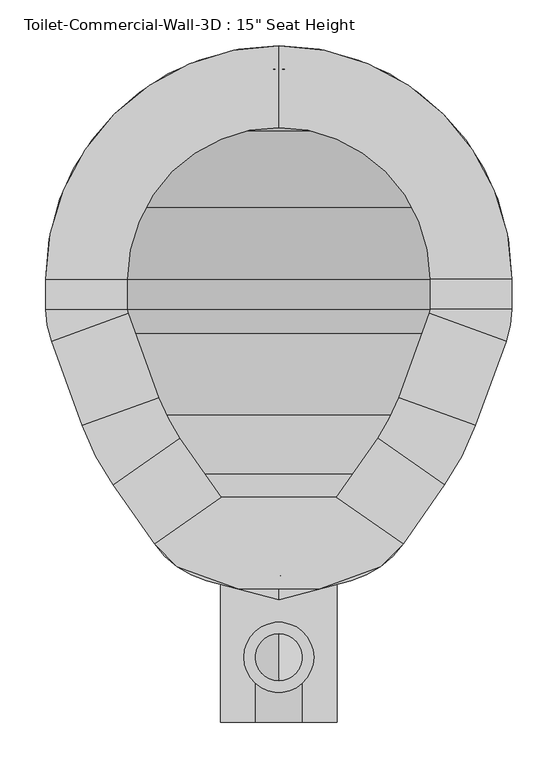
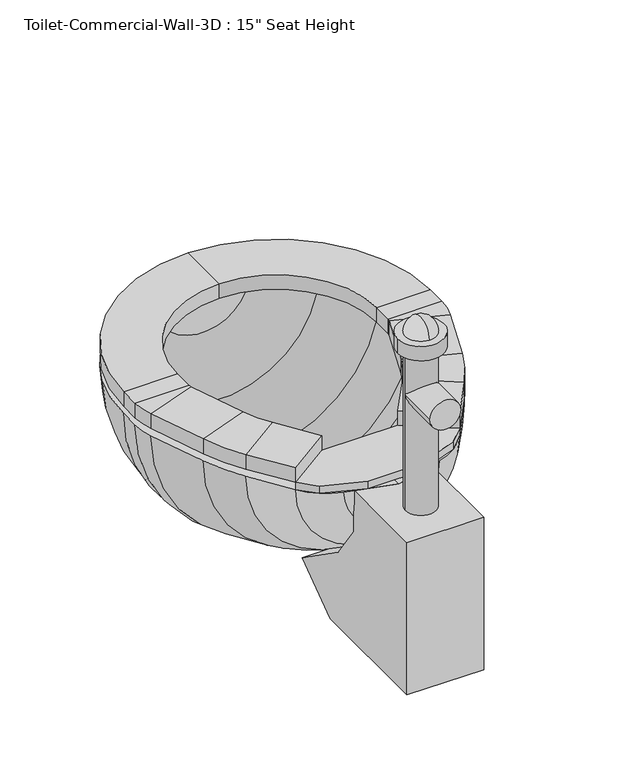
"""IFC4 building model written with IfcOpenShell, lengths in millimetres: flow terminal geometry."""

from ifc_helpers import new_model, si_unit, point, frame, frame_2d, origin, place, context, project, spatial, polyline, circle_curve, ellipse_curve, trimmed, segment, composite_curve, outline, extrude, source, transform, mapped, element, save
from ifc_brep_helpers import plane_surface, cylinder_surface, revolved_surface, advanced_brep


def flow_terminal_bd37145e(model_context):
    return source(origin(), model_context, "Body", "SolidModel", [
        extrude(outline(polyline([(467.7541169, 346.6347495), (540.5767337, 295.6438043), (515.6262519, 270.6933226), (449.563909, 246.6485961), (360.2423986, 246.6485961), (294.1800557, 270.6933226), (269.229574, 295.6438043), (342.0521907, 346.6347495), (467.7541169, 346.6347495)])), frame((0.0, 0.0, 342.9), z_axis=(0.0, 0.0, 1.0), x_axis=(1.0, 0.0, 0.0)), (0.0, 0.0, 1.0), 12.7),
        advanced_brep(
        [(467.7541169, 346.6347495, 355.6), (540.5767337, 295.6438043, 355.6), (540.5767337, 295.6438043, 381.0), (467.7541169, 346.6347495, 381.0), (512.8583992, 411.0503403, 355.6), (585.6810159, 360.0593951, 355.6), (585.6810159, 360.0593951, 381.0), (512.8583992, 411.0503403, 381.0), (619.360053, 424.7562234, 355.6), (535.821379, 455.1618141, 355.6), (619.360053, 424.7562234, 381.0), (535.821379, 455.1618141, 381.0), (569.2372501, 546.9711654, 355.6), (652.7759241, 516.5655747, 355.6), (652.7759241, 516.5655747, 381.0), (569.2372501, 546.9711654, 381.0), (658.9031538, 551.3148212, 355.6), (570.0031538, 551.3148212, 355.6), (658.9031538, 551.3148212, 381.0), (570.0031538, 551.3148212, 381.0), (570.0031538, 584.2, 355.6), (658.9031538, 584.2, 355.6), (658.9031538, 584.2, 381.0), (570.0031538, 584.2, 381.0), (404.9031538, 838.2, 355.6), (404.9031538, 749.3, 355.6), (404.9031538, 838.2, 381.0), (404.9031538, 749.3, 381.0), (150.9031538, 584.2, 355.6), (239.8031538, 584.2, 355.6), (150.9031538, 584.2, 381.0), (239.8031538, 584.2, 381.0), (239.8031538, 551.3148212, 355.6), (150.9031538, 551.3148212, 355.6), (150.9031538, 551.3148212, 381.0), (239.8031538, 551.3148212, 381.0), (157.0303835, 516.5655747, 355.6), (240.5690575, 546.9711654, 355.6), (157.0303835, 516.5655747, 381.0), (240.5690575, 546.9711654, 381.0), (273.9849286, 455.1618141, 355.6), (190.4462546, 424.7562234, 355.6), (190.4462546, 424.7562234, 381.0), (273.9849286, 455.1618141, 381.0), (224.1252917, 360.0593951, 355.6), (296.9479084, 411.0503403, 355.6), (224.1252917, 360.0593951, 381.0), (296.9479084, 411.0503403, 381.0), (342.0521907, 346.6347495, 355.6), (342.0521907, 346.6347495, 381.0), (269.229574, 295.6438043, 381.0), (269.229574, 295.6438043, 355.6)],
        [
            (0, 1),
            (1, 2),
            (2, 3),
            (3, 0),
            (0, 4),
            (4, 5),
            (5, 1),
            (5, 6),
            (6, 2),
            (6, 7),
            (7, 3),
            (7, 4),
            (8, 5, circle_curve(frame((356.8099347, 520.3166514, 355.6), z_axis=(0.0, 0.0, -1.0), x_axis=(0.81915204428899, -0.5735764363510486, 0.0)), 279.4)),
            (4, 9, circle_curve(frame((356.8099347, 520.3166514, 355.6), z_axis=(0.0, 0.0, 1.0), x_axis=(0.81915204428899, -0.5735764363510486, 0.0)), 190.5)),
            (9, 8),
            (10, 6, circle_curve(frame((356.8099347, 520.3166514, 381.0), z_axis=(0.0, 0.0, -1.0), x_axis=(0.81915204428899, -0.5735764363510486, 0.0)), 279.4)),
            (8, 10),
            (11, 7, circle_curve(frame((356.8099347, 520.3166514, 381.0), z_axis=(0.0, 0.0, -1.0), x_axis=(0.81915204428899, -0.5735764363510486, 0.0)), 190.5)),
            (10, 11),
            (11, 9),
            (9, 12),
            (12, 13),
            (13, 8),
            (13, 14),
            (14, 10),
            (14, 15),
            (15, 11),
            (15, 12),
            (16, 13, circle_curve(frame((557.3031538, 551.3148212, 355.6), z_axis=(0.0, 0.0, -1.0), x_axis=(0.939692620785906, -0.34202014332567526, 0.0)), 101.6)),
            (12, 17, circle_curve(frame((557.3031538, 551.3148212, 355.6), z_axis=(0.0, 0.0, 1.0), x_axis=(0.939692620785906, -0.34202014332567526, 0.0)), 12.7)),
            (17, 16),
            (18, 14, circle_curve(frame((557.3031538, 551.3148212, 381.0), z_axis=(0.0, 0.0, -1.0), x_axis=(0.939692620785906, -0.34202014332567526, 0.0)), 101.6)),
            (16, 18),
            (19, 15, circle_curve(frame((557.3031538, 551.3148212, 381.0), z_axis=(0.0, 0.0, -1.0), x_axis=(0.939692620785906, -0.34202014332567526, 0.0)), 12.7)),
            (18, 19),
            (19, 17),
            (17, 20),
            (20, 21),
            (21, 16),
            (21, 22),
            (22, 18),
            (22, 23),
            (23, 19),
            (23, 20),
            (24, 21, circle_curve(frame((404.9031538, 584.2, 355.6), z_axis=(0.0, 0.0, -1.0), x_axis=(1.0, 0.0, 0.0)), 254.0)),
            (20, 25, circle_curve(frame((404.9031538, 584.2, 355.6), z_axis=(0.0, 0.0, 1.0), x_axis=(1.0, 0.0, 0.0)), 165.1)),
            (25, 24),
            (26, 22, circle_curve(frame((404.9031538, 584.2, 381.0), z_axis=(0.0, 0.0, -1.0), x_axis=(1.0, 0.0, 0.0)), 254.0)),
            (24, 26),
            (27, 23, circle_curve(frame((404.9031538, 584.2, 381.0), z_axis=(0.0, 0.0, -1.0), x_axis=(1.0, 0.0, 0.0)), 165.1)),
            (26, 27),
            (27, 25),
            (28, 24, circle_curve(frame((404.9031538, 584.2, 355.6), z_axis=(0.0, 0.0, -1.0), x_axis=(0.0, 1.0, 0.0)), 254.0)),
            (25, 29, circle_curve(frame((404.9031538, 584.2, 355.6), z_axis=(0.0, 0.0, 1.0), x_axis=(0.0, 1.0, 0.0)), 165.1)),
            (29, 28),
            (30, 26, circle_curve(frame((404.9031538, 584.2, 381.0), z_axis=(0.0, 0.0, -1.0), x_axis=(0.0, 1.0, 0.0)), 254.0)),
            (28, 30),
            (31, 27, circle_curve(frame((404.9031538, 584.2, 381.0), z_axis=(0.0, 0.0, -1.0), x_axis=(0.0, 1.0, 0.0)), 165.1)),
            (30, 31),
            (31, 29),
            (29, 32),
            (32, 33),
            (33, 28),
            (33, 34),
            (34, 30),
            (34, 35),
            (35, 31),
            (35, 32),
            (36, 33, circle_curve(frame((252.5031538, 551.3148212, 355.6), z_axis=(0.0, 0.0, -1.0), x_axis=(-1.0, 0.0, 0.0)), 101.6)),
            (32, 37, circle_curve(frame((252.5031538, 551.3148212, 355.6), z_axis=(0.0, 0.0, 1.0), x_axis=(-1.0, 0.0, 0.0)), 12.7)),
            (37, 36),
            (38, 34, circle_curve(frame((252.5031538, 551.3148212, 381.0), z_axis=(0.0, 0.0, -1.0), x_axis=(-1.0, 0.0, 0.0)), 101.6)),
            (36, 38),
            (39, 35, circle_curve(frame((252.5031538, 551.3148212, 381.0), z_axis=(0.0, 0.0, -1.0), x_axis=(-1.0, 0.0, 0.0)), 12.7)),
            (38, 39),
            (39, 37),
            (37, 40),
            (40, 41),
            (41, 36),
            (41, 42),
            (42, 38),
            (42, 43),
            (43, 39),
            (43, 40),
            (44, 41, circle_curve(frame((452.9963729, 520.3166514, 355.6), z_axis=(0.0, 0.0, -1.0), x_axis=(-0.9396926207859088, -0.34202014332566766, 0.0)), 279.4)),
            (40, 45, circle_curve(frame((452.9963729, 520.3166514, 355.6), z_axis=(0.0, 0.0, 1.0), x_axis=(-0.9396926207859088, -0.34202014332566766, 0.0)), 190.5)),
            (45, 44),
            (46, 42, circle_curve(frame((452.9963729, 520.3166514, 381.0), z_axis=(0.0, 0.0, -1.0), x_axis=(-0.9396926207859088, -0.34202014332566766, 0.0)), 279.4)),
            (44, 46),
            (47, 43, circle_curve(frame((452.9963729, 520.3166514, 381.0), z_axis=(0.0, 0.0, -1.0), x_axis=(-0.9396926207859088, -0.34202014332566766, 0.0)), 190.5)),
            (46, 47),
            (47, 45),
            (48, 49),
            (49, 50),
            (50, 51),
            (51, 48),
            (45, 48),
            (51, 44),
            (50, 46),
            (49, 47),
        ],
        [
            plane_surface(frame((540.5767337, 295.6438043, 439.6203184), z_axis=(-0.5735764363510379, -0.8191520442889975, 0.0), x_axis=(0.8191520442889975, -0.5735764363510379, 0.0))),
            plane_surface(frame((467.7541169, 346.6347495, 355.6), z_axis=(0.0, 0.0, -1.0), x_axis=(0.5735764363510375, 0.8191520442889978, 0.0))),
            plane_surface(frame((540.5767337, 295.6438043, 355.6), z_axis=(0.8191520442889973, -0.5735764363510383, 0.0), x_axis=(0.5735764363510383, 0.8191520442889973, 0.0))),
            plane_surface(frame((540.5767337, 295.6438043, 381.0), z_axis=(0.0, 0.0, 1.0), x_axis=(0.573576436351038, 0.8191520442889975, 0.0))),
            plane_surface(frame((467.7541169, 346.6347495, 381.0), z_axis=(-0.8191520442889981, 0.5735764363510371, 0.0), x_axis=(0.5735764363510371, 0.8191520442889981, 0.0))),
            plane_surface(frame((356.8099347, 520.3166514, 355.6), z_axis=(0.0, 0.0, -1.0), x_axis=(0.81915204428899, -0.5735764363510486, 0.0))),
            cylinder_surface(frame((356.8099347, 520.3166514, 342.9), z_axis=(0.0, 0.0, 1.0), x_axis=(0.81915204428899, -0.5735764363510486, 0.0)), 279.4),
            plane_surface(frame((356.8099347, 520.3166514, 381.0), z_axis=(0.0, 0.0, 1.0), x_axis=(0.81915204428899, -0.5735764363510486, 0.0))),
            revolved_surface(polyline([(512.8583991370526, 411.0503402751252, 381.0), (512.8583991370526, 411.0503402751252, 355.6)]), (356.8099347, 520.3166514, 342.9), (0.0, 0.0, 1.0)),
            plane_surface(frame((535.821379, 455.1618141, 355.6), z_axis=(0.0, 0.0, -1.0), x_axis=(0.3420201433256632, 0.9396926207859104, 0.0))),
            plane_surface(frame((619.360053, 424.7562234, 355.6), z_axis=(0.9396926207859108, -0.34202014332566233, 0.0), x_axis=(0.34202014332566233, 0.9396926207859108, 0.0))),
            plane_surface(frame((619.360053, 424.7562234, 381.0), z_axis=(0.0, 0.0, 1.0), x_axis=(0.3420201433256635, 0.9396926207859103, 0.0))),
            plane_surface(frame((535.821379, 455.1618141, 381.0), z_axis=(-0.9396926207859103, 0.3420201433256636, 0.0), x_axis=(0.3420201433256636, 0.9396926207859103, 0.0))),
            plane_surface(frame((557.3031538, 551.3148212, 355.6), z_axis=(0.0, 0.0, -1.0), x_axis=(0.939692620785906, -0.34202014332567526, 0.0))),
            cylinder_surface(frame((557.3031538, 551.3148212, 342.9), z_axis=(0.0, 0.0, 1.0), x_axis=(0.939692620785906, -0.34202014332567526, 0.0)), 101.6),
            plane_surface(frame((557.3031538, 551.3148212, 381.0), z_axis=(0.0, 0.0, 1.0), x_axis=(0.939692620785906, -0.34202014332567526, 0.0))),
            revolved_surface(polyline([(569.237250083981, 546.9711653797639, 381.0), (569.237250083981, 546.9711653797639, 355.6)]), (557.3031538, 551.3148212, 342.9), (0.0, 0.0, 1.0)),
            plane_surface(frame((570.0031538, 551.3148212, 355.6), z_axis=(0.0, 0.0, -1.0), x_axis=(0.0, 1.0, 0.0))),
            plane_surface(frame((658.9031538, 551.3148212, 355.6), z_axis=(1.0, 0.0, 0.0), x_axis=(0.0, 1.0, 0.0))),
            plane_surface(frame((658.9031538, 551.3148212, 381.0), z_axis=(0.0, 0.0, 1.0), x_axis=(0.0, 1.0, 0.0))),
            plane_surface(frame((570.0031538, 551.3148212, 381.0), z_axis=(-1.0, 0.0, 0.0), x_axis=(0.0, 1.0, 0.0))),
            plane_surface(frame((404.9031538, 584.2, 355.6), z_axis=(0.0, 0.0, -1.0), x_axis=(1.0, 0.0, 0.0))),
            cylinder_surface(frame((404.9031538, 584.2, 342.9), z_axis=(0.0, 0.0, 1.0), x_axis=(1.0, 0.0, 0.0)), 254.0),
            plane_surface(frame((404.9031538, 584.2, 381.0), z_axis=(0.0, 0.0, 1.0), x_axis=(1.0, 0.0, 0.0))),
            revolved_surface(polyline([(570.0031538, 584.2, 381.0), (570.0031538, 584.2, 355.6)]), (404.9031538, 584.2, 342.9), (0.0, 0.0, 1.0)),
            plane_surface(frame((404.9031538, 584.2, 355.6), z_axis=(0.0, 0.0, -1.0), x_axis=(0.0, 1.0, 0.0))),
            cylinder_surface(frame((404.9031538, 584.2, 342.9), z_axis=(0.0, 0.0, 1.0), x_axis=(0.0, 1.0, 0.0)), 254.0),
            plane_surface(frame((404.9031538, 584.2, 381.0), z_axis=(0.0, 0.0, 1.0), x_axis=(0.0, 1.0, 0.0))),
            revolved_surface(polyline([(404.9031538, 749.3000000000001, 381.0), (404.9031538, 749.3000000000001, 355.6)]), (404.9031538, 584.2, 342.9), (0.0, 0.0, 1.0)),
            plane_surface(frame((239.8031538, 584.2, 355.6), z_axis=(0.0, 0.0, -1.0), x_axis=(0.0, -1.0, 0.0))),
            plane_surface(frame((150.9031538, 584.2, 355.6), z_axis=(-1.0, 0.0, 0.0), x_axis=(0.0, -1.0, 0.0))),
            plane_surface(frame((150.9031538, 584.2, 381.0), z_axis=(0.0, 0.0, 1.0), x_axis=(0.0, -1.0, 0.0))),
            plane_surface(frame((239.8031538, 584.2, 381.0), z_axis=(1.0, 0.0, 0.0), x_axis=(0.0, -1.0, 0.0))),
            plane_surface(frame((252.5031538, 551.3148212, 355.6), z_axis=(0.0, 0.0, -1.0), x_axis=(-1.0, 0.0, 0.0))),
            cylinder_surface(frame((252.5031538, 551.3148212, 342.9), z_axis=(0.0, 0.0, 1.0), x_axis=(-1.0, 0.0, 0.0)), 101.6),
            plane_surface(frame((252.5031538, 551.3148212, 381.0), z_axis=(0.0, 0.0, 1.0), x_axis=(-1.0, 0.0, 0.0))),
            revolved_surface(polyline([(239.80315380000002, 551.3148212, 381.0), (239.80315380000002, 551.3148212, 355.6)]), (252.5031538, 551.3148212, 342.9), (0.0, 0.0, 1.0)),
            plane_surface(frame((240.5690575, 546.9711654, 355.6), z_axis=(0.0, 0.0, -1.0), x_axis=(0.3420201433256559, -0.9396926207859131, 0.0))),
            plane_surface(frame((157.0303835, 516.5655747, 355.6), z_axis=(-0.9396926207859132, -0.34202014332565567, 0.0), x_axis=(0.34202014332565567, -0.9396926207859132, 0.0))),
            plane_surface(frame((157.0303835, 516.5655747, 381.0), z_axis=(0.0, 0.0, 1.0), x_axis=(0.34202014332565556, -0.9396926207859132, 0.0))),
            plane_surface(frame((240.5690575, 546.9711654, 381.0), z_axis=(0.9396926207859131, 0.34202014332565583, 0.0), x_axis=(0.34202014332565583, -0.9396926207859131, 0.0))),
            plane_surface(frame((452.9963729, 520.3166514, 355.6), z_axis=(0.0, 0.0, -1.0), x_axis=(-0.9396926207859088, -0.34202014332566766, 0.0))),
            cylinder_surface(frame((452.9963729, 520.3166514, 342.9), z_axis=(0.0, 0.0, 1.0), x_axis=(-0.9396926207859088, -0.34202014332566766, 0.0)), 279.4),
            plane_surface(frame((452.9963729, 520.3166514, 381.0), z_axis=(0.0, 0.0, 1.0), x_axis=(-0.9396926207859088, -0.34202014332566766, 0.0))),
            revolved_surface(polyline([(273.98492864028435, 455.16181409646026, 381.0), (273.98492864028435, 455.16181409646026, 355.6)]), (452.9963729, 520.3166514, 342.9), (0.0, 0.0, 1.0)),
            plane_surface(frame((269.229574, 295.6438043, 246.1796816), z_axis=(0.5735764363510504, -0.8191520442889889, 0.0), x_axis=(0.8191520442889889, 0.5735764363510504, 0.0))),
            plane_surface(frame((296.9479084, 411.0503403, 355.6), z_axis=(0.0, 0.0, -1.0000000000000002), x_axis=(0.5735764363510502, -0.819152044288989, 0.0))),
            plane_surface(frame((224.1252917, 360.0593951, 355.6), z_axis=(-0.819152044288989, -0.5735764363510502, 0.0), x_axis=(0.5735764363510502, -0.819152044288989, 0.0))),
            plane_surface(frame((224.1252917, 360.0593951, 381.0), z_axis=(0.0, 0.0, 1.0), x_axis=(0.5735764363510496, -0.8191520442889894, 0.0))),
            plane_surface(frame((296.9479084, 411.0503403, 381.0), z_axis=(0.8191520442889881, 0.5735764363510514, 0.0), x_axis=(0.5735764363510514, -0.8191520442889881, 0.0))),
        ],
        [
            (0, [[1, 2, 3, 4]]),
            (1, [[-1, 5, 6, 7]]),
            (2, [[-2, -7, 8, 9]]),
            (3, [[-3, -9, 10, 11]]),
            (4, [[-4, -11, 12, -5]]),
            (5, [[13, -6, 14, 15]]),
            (6, [[16, -8, -13, 17]]),
            (7, [[18, -10, -16, 19]]),
            (8, [[-14, -12, -18, 20]]),
            (9, [[-15, 21, 22, 23]]),
            (10, [[-17, -23, 24, 25]]),
            (11, [[-19, -25, 26, 27]]),
            (12, [[-20, -27, 28, -21]]),
            (13, [[29, -22, 30, 31]]),
            (14, [[32, -24, -29, 33]]),
            (15, [[34, -26, -32, 35]]),
            (16, [[-30, -28, -34, 36]]),
            (17, [[-31, 37, 38, 39]]),
            (18, [[-33, -39, 40, 41]]),
            (19, [[-35, -41, 42, 43]]),
            (20, [[-36, -43, 44, -37]]),
            (21, [[45, -38, 46, 47]]),
            (22, [[48, -40, -45, 49]]),
            (23, [[50, -42, -48, 51]]),
            (24, [[-46, -44, -50, 52]]),
            (25, [[53, -47, 54, 55]]),
            (26, [[56, -49, -53, 57]]),
            (27, [[58, -51, -56, 59]]),
            (28, [[-54, -52, -58, 60]]),
            (29, [[-55, 61, 62, 63]]),
            (30, [[-57, -63, 64, 65]]),
            (31, [[-59, -65, 66, 67]]),
            (32, [[-60, -67, 68, -61]]),
            (33, [[69, -62, 70, 71]]),
            (34, [[72, -64, -69, 73]]),
            (35, [[74, -66, -72, 75]]),
            (36, [[-70, -68, -74, 76]]),
            (37, [[-71, 77, 78, 79]]),
            (38, [[-73, -79, 80, 81]]),
            (39, [[-75, -81, 82, 83]]),
            (40, [[-76, -83, 84, -77]]),
            (41, [[85, -78, 86, 87]]),
            (42, [[88, -80, -85, 89]]),
            (43, [[90, -82, -88, 91]]),
            (44, [[-86, -84, -90, 92]]),
            (45, [[93, 94, 95, 96]]),
            (46, [[-87, 97, -96, 98]]),
            (47, [[-89, -98, -95, 99]]),
            (48, [[-91, -99, -94, 100]]),
            (49, [[-92, -100, -93, -97]]),
        ],
    ),
        advanced_brep(
        [(491.7762702, 822.8819257, 342.9), (404.9031538, 838.2, 342.9), (404.9031538, 812.8, 342.9), (483.0889586, 799.0137331, 342.9), (566.547764, 745.8446102, 342.9), (619.7168869, 662.3858048, 342.9), (633.5031538, 584.2, 342.9), (633.5031538, 551.3148212, 342.9), (628.9077315, 525.2528863, 342.9), (596.6355667, 436.5858422, 342.9), (562.9565296, 371.8890139, 342.9), (525.0728964, 317.7855786, 342.9), (468.1430637, 277.9228806, 342.9), (404.9031538, 260.9777978, 342.9), (404.9031538, 234.6817829, 342.9), (483.6469009, 255.7811063, 342.9), (540.5767337, 295.6438043, 342.9), (585.6810159, 360.0593951, 342.9), (619.360053, 424.7562234, 342.9), (652.7759241, 516.5655747, 342.9), (658.9031538, 551.3148212, 342.9), (658.9031538, 584.2, 342.9), (643.5850795, 671.0731164, 342.9), (584.5082762, 763.8051224, 342.9), (318.0300374, 822.8819257, 342.9), (225.2980314, 763.8051224, 342.9), (166.2212281, 671.0731164, 342.9), (150.9031538, 584.2, 342.9), (150.9031538, 551.3148212, 342.9), (157.0303835, 516.5655747, 342.9), (190.4462546, 424.7562234, 342.9), (224.1252917, 360.0593951, 342.9), (269.229574, 295.6438043, 342.9), (326.1594067, 255.7811063, 342.9), (341.663244, 277.9228806, 342.9), (284.7334112, 317.7855786, 342.9), (246.849778, 371.8890139, 342.9), (213.1707409, 436.5858422, 342.9), (180.8985761, 525.2528863, 342.9), (176.3031538, 551.3148212, 342.9), (176.3031538, 584.2, 342.9), (190.0894207, 662.3858048, 342.9), (243.2585436, 745.8446102, 342.9), (326.7173491, 799.0137331, 342.9)],
        [
            (0, 1, circle_curve(frame((404.9031538, 584.2, 342.9), z_axis=(0.0, 0.0, 1.0), x_axis=(1.0, 0.0, 0.0)), 254.0)),
            (1, 2),
            (2, 3, circle_curve(frame((404.9031538, 584.2, 342.9), z_axis=(0.0, 0.0, -1.0), x_axis=(1.0, 0.0, 0.0)), 228.6)),
            (3, 4, circle_curve(frame((404.9031538, 584.2, 342.9), z_axis=(0.0, 0.0, -1.0), x_axis=(1.0, 0.0, 0.0)), 228.6)),
            (4, 5, circle_curve(frame((404.9031538, 584.2, 342.9), z_axis=(0.0, 0.0, -1.0), x_axis=(1.0, 0.0, 0.0)), 228.6)),
            (5, 6, circle_curve(frame((404.9031538, 584.2, 342.9), z_axis=(0.0, 0.0, -1.0), x_axis=(1.0, 0.0, 0.0)), 228.6)),
            (6, 7),
            (7, 8, circle_curve(frame((557.3031538, 551.3148212, 342.9), z_axis=(0.0, 0.0, -1.0), x_axis=(1.0, 0.0, 0.0)), 76.2)),
            (8, 9),
            (9, 10, circle_curve(frame((334.0854485, 532.1462703, 342.9), z_axis=(0.0, 0.0, -1.0), x_axis=(1.0, 0.0, 0.0)), 279.4)),
            (10, 11),
            (11, 12, circle_curve(frame((441.8470487, 376.0609446, 342.9), z_axis=(0.0, 0.0, -1.0), x_axis=(1.0, 0.0, 0.0)), 101.6)),
            (12, 13),
            (13, 14),
            (14, 15),
            (15, 16, circle_curve(frame((457.350886, 353.9191703, 342.9), z_axis=(0.0, 0.0, 1.0), x_axis=(1.0, 0.0, 0.0)), 101.6)),
            (16, 17),
            (17, 18, circle_curve(frame((356.8099347, 520.3166514, 342.9), z_axis=(0.0, 0.0, 1.0), x_axis=(1.0, 0.0, 0.0)), 279.4)),
            (18, 19),
            (19, 20, circle_curve(frame((557.3031538, 551.3148212, 342.9), z_axis=(0.0, 0.0, 1.0), x_axis=(1.0, 0.0, 0.0)), 101.6)),
            (20, 21),
            (21, 22, circle_curve(frame((404.9031538, 584.2, 342.9), z_axis=(0.0, 0.0, 1.0), x_axis=(1.0, 0.0, 0.0)), 254.0)),
            (22, 23, circle_curve(frame((404.9031538, 584.2, 342.9), z_axis=(0.0, 0.0, 1.0), x_axis=(1.0, 0.0, 0.0)), 254.0)),
            (23, 0, circle_curve(frame((404.9031538, 584.2, 342.9), z_axis=(0.0, 0.0, 1.0), x_axis=(1.0, 0.0, 0.0)), 254.0)),
            (24, 25, circle_curve(frame((404.9031538, 584.2, 342.9), z_axis=(0.0, 0.0, 1.0), x_axis=(-1.0, 0.0, 0.0)), 254.0)),
            (25, 26, circle_curve(frame((404.9031538, 584.2, 342.9), z_axis=(0.0, 0.0, 1.0), x_axis=(-1.0, 0.0, 0.0)), 254.0)),
            (26, 27, circle_curve(frame((404.9031538, 584.2, 342.9), z_axis=(0.0, 0.0, 1.0), x_axis=(-1.0, 0.0, 0.0)), 254.0)),
            (27, 28),
            (28, 29, circle_curve(frame((252.5031538, 551.3148212, 342.9), z_axis=(0.0, 0.0, 1.0), x_axis=(-1.0, 0.0, 0.0)), 101.6)),
            (29, 30),
            (30, 31, circle_curve(frame((452.9963729, 520.3166514, 342.9), z_axis=(0.0, 0.0, 1.0), x_axis=(-1.0, 0.0, 0.0)), 279.4)),
            (31, 32),
            (32, 33, circle_curve(frame((352.4554217, 353.9191703, 342.9), z_axis=(0.0, 0.0, 1.0), x_axis=(-1.0, 0.0, 0.0)), 101.6)),
            (33, 14),
            (13, 34),
            (34, 35, circle_curve(frame((367.9592589, 376.0609446, 342.9), z_axis=(0.0, 0.0, -1.0), x_axis=(-1.0, 0.0, 0.0)), 101.6)),
            (35, 36),
            (36, 37, circle_curve(frame((475.7208592, 532.1462703, 342.9), z_axis=(0.0, 0.0, -1.0), x_axis=(-1.0, 0.0, 0.0)), 279.4)),
            (37, 38),
            (38, 39, circle_curve(frame((252.5031538, 551.3148212, 342.9), z_axis=(0.0, 0.0, -1.0), x_axis=(-1.0, 0.0, 0.0)), 76.2)),
            (39, 40),
            (40, 41, circle_curve(frame((404.9031538, 584.2, 342.9), z_axis=(0.0, 0.0, -1.0), x_axis=(-1.0, 0.0, 0.0)), 228.6)),
            (41, 42, circle_curve(frame((404.9031538, 584.2, 342.9), z_axis=(0.0, 0.0, -1.0), x_axis=(-1.0, 0.0, 0.0)), 228.6)),
            (42, 43, circle_curve(frame((404.9031538, 584.2, 342.9), z_axis=(0.0, 0.0, -1.0), x_axis=(-1.0, 0.0, 0.0)), 228.6)),
            (43, 2, circle_curve(frame((404.9031538, 584.2, 342.9), z_axis=(0.0, 0.0, -1.0), x_axis=(-1.0, 0.0, 0.0)), 228.6)),
            (1, 24, circle_curve(frame((404.9031538, 584.2, 342.9), z_axis=(0.0, 0.0, 1.0), x_axis=(-1.0, 0.0, 0.0)), 254.0)),
            (0, 24, circle_curve(frame((404.9031538, 822.8819257, 342.9), z_axis=(0.0, 1.0, 0.0), x_axis=(1.0, 0.0, 0.0)), 86.8731164)),
            (43, 3, circle_curve(frame((404.9031538, 799.0137331, 342.9), z_axis=(0.0, -1.0, 0.0), x_axis=(1.0, 0.0, 0.0)), 78.1858048)),
            (42, 4, circle_curve(frame((404.9031538, 745.8446102, 342.9), z_axis=(0.0, -1.0, 0.0), x_axis=(1.0, 0.0, 0.0)), 161.6446102)),
            (41, 5, circle_curve(frame((404.9031538, 662.3858048, 342.9), z_axis=(0.0, -1.0, 0.0), x_axis=(1.0, 0.0, 0.0)), 214.8137331)),
            (40, 6, circle_curve(frame((404.9031538, 584.2, 342.9), z_axis=(0.0, -1.0, 0.0), x_axis=(1.0, 0.0, 0.0)), 228.6)),
            (39, 7, circle_curve(frame((404.9031538, 551.3148212, 342.9), z_axis=(0.0, -1.0, 0.0), x_axis=(1.0, 0.0, 0.0)), 228.6)),
            (38, 8, circle_curve(frame((404.9031538, 525.2528863, 342.9), z_axis=(0.0, -1.0, 0.0), x_axis=(1.0, 0.0, 0.0)), 224.0045777)),
            (37, 9, circle_curve(frame((404.9031538, 436.5858422, 342.9), z_axis=(0.0, -1.0, 0.0), x_axis=(1.0, 0.0, 0.0)), 191.7324129)),
            (36, 10, circle_curve(frame((404.9031538, 371.8890139, 342.9), z_axis=(0.0, -1.0, 0.0), x_axis=(1.0, 0.0, 0.0)), 158.0533758)),
            (35, 11, circle_curve(frame((404.9031538, 317.7855786, 342.9), z_axis=(0.0, -1.0, 0.0), x_axis=(1.0, 0.0, 0.0)), 120.1697426)),
            (34, 12, circle_curve(frame((404.9031538, 277.9228806, 342.9), z_axis=(0.0, -1.0, 0.0), x_axis=(1.0, 0.0, 0.0)), 63.2399099)),
            (33, 15, circle_curve(frame((404.9031538, 255.7811063, 342.9), z_axis=(0.0, -1.0, 0.0), x_axis=(1.0, 0.0, 0.0)), 78.7437471)),
            (32, 16, circle_curve(frame((404.9031538, 295.6438043, 342.9), z_axis=(0.0, -1.0, 0.0), x_axis=(1.0, 0.0, 0.0)), 135.6735798)),
            (31, 17, circle_curve(frame((404.9031538, 360.0593951, 342.9), z_axis=(0.0, -1.0, 0.0), x_axis=(1.0, 0.0, 0.0)), 180.7778621)),
            (30, 18, circle_curve(frame((404.9031538, 424.7562234, 342.9), z_axis=(0.0, -1.0, 0.0), x_axis=(1.0, 0.0, 0.0)), 214.4568992)),
            (29, 19, circle_curve(frame((404.9031538, 516.5655747, 342.9), z_axis=(0.0, -1.0, 0.0), x_axis=(1.0, 0.0, 0.0)), 247.8727703)),
            (28, 20, circle_curve(frame((404.9031538, 551.3148212, 342.9), z_axis=(0.0, -1.0, 0.0), x_axis=(1.0, 0.0, 0.0)), 254.0)),
            (27, 21, circle_curve(frame((404.9031538, 584.2, 342.9), z_axis=(0.0, -1.0, 0.0), x_axis=(1.0, 0.0, 0.0)), 254.0)),
            (26, 22, circle_curve(frame((404.9031538, 671.0731164, 342.9), z_axis=(0.0, -1.0, 0.0), x_axis=(1.0, 0.0, 0.0)), 238.6819257)),
            (25, 23, circle_curve(frame((404.9031538, 763.8051224, 342.9), z_axis=(0.0, -1.0, 0.0), x_axis=(1.0, 0.0, 0.0)), 179.6051224)),
        ],
        [
            plane_surface(frame((404.9031538, 943.4102448, 342.9), z_axis=(0.0, 0.0, 1.0), x_axis=(1.0, 0.0, 0.0))),
            plane_surface(frame((404.9031538, 943.4102448, 342.9), z_axis=(0.0, 0.0, 1.0), x_axis=(-1.0, 0.0, 0.0))),
            revolved_surface(trimmed(ellipse_curve(frame((404.9031538, 584.2, 342.9), z_axis=(0.0, 0.0, 1.0), x_axis=(1.0, 0.0, 0.0)), 254.0, 254.0), [point((491.7762702, 822.8819257, 342.9))], [point((404.9031538, 838.2, 342.9))], True, "CARTESIAN"), (404.9031538, 943.4102448, 342.9), (0.0, 1.0, 0.0)),
            revolved_surface(trimmed(ellipse_curve(frame((404.9031538, 584.2, 342.9), z_axis=(0.0, 0.0, -1.0), x_axis=(1.0, 0.0, 0.0)), 228.6, 228.6), [point((404.9031538, 812.8, 342.9))], [point((483.0889586, 799.0137331, 342.9))], True, "CARTESIAN"), (404.9031538, 943.4102448, 342.9), (0.0, 1.0, 0.0)),
            revolved_surface(trimmed(ellipse_curve(frame((404.9031538, 584.2, 342.9), z_axis=(0.0, 0.0, -1.0), x_axis=(1.0, 0.0, 0.0)), 228.6, 228.6), [point((483.0889586, 799.0137331, 342.9))], [point((566.547764, 745.8446102, 342.9))], True, "CARTESIAN"), (404.9031538, 943.4102448, 342.9), (0.0, 1.0, 0.0)),
            revolved_surface(trimmed(ellipse_curve(frame((404.9031538, 584.2, 342.9), z_axis=(0.0, 0.0, -1.0), x_axis=(1.0, 0.0, 0.0)), 228.6, 228.6), [point((566.547764, 745.8446102, 342.9))], [point((619.7168869, 662.3858048, 342.9))], True, "CARTESIAN"), (404.9031538, 943.4102448, 342.9), (0.0, 1.0, 0.0)),
            revolved_surface(trimmed(ellipse_curve(frame((404.9031538, 584.2, 342.9), z_axis=(0.0, 0.0, -1.0), x_axis=(1.0, 0.0, 0.0)), 228.6, 228.6), [point((619.7168869, 662.3858048, 342.9))], [point((633.5031538, 584.2, 342.9))], True, "CARTESIAN"), (404.9031538, 943.4102448, 342.9), (0.0, 1.0, 0.0)),
            revolved_surface(polyline([(633.5031538, 584.2, 342.9), (633.5031538, 551.3148212, 342.9)]), (404.9031538, 943.4102448, 342.9), (0.0, 1.0, 0.0)),
            revolved_surface(trimmed(ellipse_curve(frame((557.3031538, 551.3148212, 342.9), z_axis=(0.0, 0.0, -1.0), x_axis=(1.0, 0.0, 0.0)), 76.2, 76.2), [point((633.5031538, 551.3148212, 342.9))], [point((628.9077315, 525.2528863, 342.9))], True, "CARTESIAN"), (404.9031538, 943.4102448, 342.9), (0.0, 1.0, 0.0)),
            revolved_surface(polyline([(628.9077315, 525.2528863, 342.9), (596.6355667, 436.5858422, 342.9)]), (404.9031538, 943.4102448, 342.9), (0.0, 1.0, 0.0)),
            revolved_surface(trimmed(ellipse_curve(frame((334.0854485, 532.1462703, 342.9), z_axis=(0.0, 0.0, -1.0), x_axis=(1.0, 0.0, 0.0)), 279.4, 279.4), [point((596.6355667, 436.5858422, 342.9))], [point((562.9565296, 371.8890139, 342.9))], True, "CARTESIAN"), (404.9031538, 943.4102448, 342.9), (0.0, 1.0, 0.0)),
            revolved_surface(polyline([(562.9565296, 371.8890139, 342.9), (525.0728964, 317.7855786, 342.9)]), (404.9031538, 943.4102448, 342.9), (0.0, 1.0, 0.0)),
            revolved_surface(trimmed(ellipse_curve(frame((441.8470487, 376.0609446, 342.9), z_axis=(0.0, 0.0, -1.0), x_axis=(1.0, 0.0, 0.0)), 101.6, 101.6), [point((525.0728964, 317.7855786, 342.9))], [point((468.1430637, 277.9228806, 342.9))], True, "CARTESIAN"), (404.9031538, 943.4102448, 342.9), (0.0, 1.0, 0.0)),
            revolved_surface(polyline([(468.1430637, 277.9228806, 342.9), (404.9031538, 260.9777978, 342.9)]), (404.9031538, 943.4102448, 342.9), (0.0, 1.0, 0.0)),
            revolved_surface(polyline([(404.9031538, 234.6817829, 342.9), (483.6469009, 255.7811063, 342.9)]), (404.9031538, 943.4102448, 342.9), (0.0, 1.0, 0.0)),
            revolved_surface(trimmed(ellipse_curve(frame((457.350886, 353.9191703, 342.9), z_axis=(0.0, 0.0, 1.0), x_axis=(1.0, 0.0, 0.0)), 101.6, 101.6), [point((483.6469009, 255.7811063, 342.9))], [point((540.5767337, 295.6438043, 342.9))], True, "CARTESIAN"), (404.9031538, 943.4102448, 342.9), (0.0, 1.0, 0.0)),
            revolved_surface(polyline([(540.5767337, 295.6438043, 342.9), (585.6810159, 360.0593951, 342.9)]), (404.9031538, 943.4102448, 342.9), (0.0, 1.0, 0.0)),
            revolved_surface(trimmed(ellipse_curve(frame((356.8099347, 520.3166514, 342.9), z_axis=(0.0, 0.0, 1.0), x_axis=(1.0, 0.0, 0.0)), 279.4, 279.4), [point((585.6810159, 360.0593951, 342.9))], [point((619.360053, 424.7562234, 342.9))], True, "CARTESIAN"), (404.9031538, 943.4102448, 342.9), (0.0, 1.0, 0.0)),
            revolved_surface(polyline([(619.360053, 424.7562234, 342.9), (652.7759241, 516.5655747, 342.9)]), (404.9031538, 943.4102448, 342.9), (0.0, 1.0, 0.0)),
            revolved_surface(trimmed(ellipse_curve(frame((557.3031538, 551.3148212, 342.9), z_axis=(0.0, 0.0, 1.0), x_axis=(1.0, 0.0, 0.0)), 101.6, 101.6), [point((652.7759241, 516.5655747, 342.9))], [point((658.9031538, 551.3148212, 342.9))], True, "CARTESIAN"), (404.9031538, 943.4102448, 342.9), (0.0, 1.0, 0.0)),
            cylinder_surface(frame((404.9031538, 943.4102448, 342.9), z_axis=(0.0, 1.0, 0.0), x_axis=(1.0, 0.0, 0.0)), 254.0),
            revolved_surface(trimmed(ellipse_curve(frame((404.9031538, 584.2, 342.9), z_axis=(0.0, 0.0, 1.0), x_axis=(1.0, 0.0, 0.0)), 254.0, 254.0), [point((658.9031538, 584.2, 342.9))], [point((643.5850795, 671.0731164, 342.9))], True, "CARTESIAN"), (404.9031538, 943.4102448, 342.9), (0.0, 1.0, 0.0)),
            revolved_surface(trimmed(ellipse_curve(frame((404.9031538, 584.2, 342.9), z_axis=(0.0, 0.0, 1.0), x_axis=(1.0, 0.0, 0.0)), 254.0, 254.0), [point((643.5850795, 671.0731164, 342.9))], [point((584.5082762, 763.8051224, 342.9))], True, "CARTESIAN"), (404.9031538, 943.4102448, 342.9), (0.0, 1.0, 0.0)),
            revolved_surface(trimmed(ellipse_curve(frame((404.9031538, 584.2, 342.9), z_axis=(0.0, 0.0, 1.0), x_axis=(1.0, 0.0, 0.0)), 254.0, 254.0), [point((584.5082762, 763.8051224, 342.9))], [point((491.7762702, 822.8819257, 342.9))], True, "CARTESIAN"), (404.9031538, 943.4102448, 342.9), (0.0, 1.0, 0.0)),
        ],
        [
            (0, [[1, 2, 3, 4, 5, 6, 7, 8, 9, 10, 11, 12, 13, 14, 15, 16, 17, 18, 19, 20, 21, 22, 23, 24]]),
            (1, [[25, 26, 27, 28, 29, 30, 31, 32, 33, 34, -14, 35, 36, 37, 38, 39, 40, 41, 42, 43, 44, 45, -2, 46]]),
            (2, [[-1, 47, -46]]),
            (3, [[48, -3, -45]]),
            (4, [[49, -4, -48, -44]]),
            (5, [[50, -5, -49, -43]]),
            (6, [[51, -6, -50, -42]]),
            (7, [[52, -7, -51, -41]]),
            (8, [[53, -8, -52, -40]]),
            (9, [[54, -9, -53, -39]]),
            (10, [[55, -10, -54, -38]]),
            (11, [[56, -11, -55, -37]]),
            (12, [[57, -12, -56, -36]]),
            (13, [[-13, -57, -35]]),
            (14, [[58, -15, -34]]),
            (15, [[59, -16, -58, -33]]),
            (16, [[60, -17, -59, -32]]),
            (17, [[61, -18, -60, -31]]),
            (18, [[62, -19, -61, -30]]),
            (19, [[63, -20, -62, -29]]),
            (20, [[64, -21, -63, -28]]),
            (21, [[65, -22, -64, -27]]),
            (22, [[66, -23, -65, -26]]),
            (23, [[-47, -24, -66, -25]]),
        ],
    ),
        advanced_brep(
        [(404.9031538, 146.5176912, 647.7), (404.9031538, 197.7528563, 647.7), (404.9031538, 172.1352737, 673.3175826), (404.9031538, 172.1352737, 647.7)],
        [
            (0, 1, circle_curve(frame((404.9031538, 172.1352737, 647.7), z_axis=(0.0, 0.0, 1.0), x_axis=(0.0, 1.0, 0.0)), 25.6175826)),
            (1, 2, circle_curve(frame((404.9031538, 172.1352737, 647.7), z_axis=(1.0, 0.0, 0.0), x_axis=(0.0, -1.0, 0.0)), 25.6175826)),
            (2, 0, circle_curve(frame((404.9031538, 172.1352737, 647.7), z_axis=(1.0, 0.0, 0.0), x_axis=(0.0, 1.0, 0.0)), 25.6175826)),
            (1, 0, circle_curve(frame((404.9031538, 172.1352737, 647.7), z_axis=(0.0, 0.0, 1.0), x_axis=(0.0, 1.0, 0.0)), 25.6175826)),
            (3, 1),
            (0, 3),
        ],
        [
            revolved_surface(trimmed(ellipse_curve(frame((404.9031538, 172.1352737, 647.7), z_axis=(-1.0, 0.0, 0.0), x_axis=(0.0, -1.0, 0.0)), 25.6175826, 25.6175826), [point((404.9031538, 172.1352737, 673.3175826))], [point((404.9031538, 197.7528563, 647.7))], True, "CARTESIAN"), (404.9031538, 172.1352737, 712.3277273), (0.0, 0.0, -1.0)),
            plane_surface(frame((404.9031538, 172.1352737, 647.7), z_axis=(0.0, 0.0, -1.0), x_axis=(0.0, 1.0, 0.0))),
        ],
        [
            (0, [[1, 2, 3]]),
            (0, [[4, -3, -2]]),
            (1, [[5, -1, 6]]),
            (1, [[-6, -4, -5]]),
        ],
    ),
        extrude(outline(composite_curve([segment(trimmed(circle_curve(frame_2d((404.9031538, 172.1352737)), 38.1), [point((366.8031538, 172.1352737))], [point((443.0031538, 172.1352737))], False, "CARTESIAN"), True, "CONTINUOUS"), segment(trimmed(circle_curve(frame_2d((404.9031538, 172.1352737)), 38.1), [point((443.0031538, 172.1352737))], [point((366.8031538, 172.1352737))], False, "CARTESIAN"), True, "CONTINUOUS")], self_intersect=False)), frame((0.0, 0.0, 622.3), z_axis=(0.0, 0.0, 1.0), x_axis=(1.0, 0.0, 0.0)), (0.0, 0.0, 1.0), 25.4),
        extrude(outline(composite_curve([segment(trimmed(circle_curve(frame_2d((544.2113641, 404.9031538)), 25.4), [point((544.2113641, 379.5031538))], [point((544.2113641, 430.3031538))], False, "CARTESIAN"), True, "CONTINUOUS"), segment(trimmed(circle_curve(frame_2d((544.2113641, 404.9031538)), 25.4), [point((544.2113641, 430.3031538))], [point((544.2113641, 379.5031538))], False, "CARTESIAN"), True, "CONTINUOUS")], self_intersect=False)), frame((0.0, 101.6, 0.0), z_axis=(0.0, 1.0, 0.0), x_axis=(0.0, 0.0, 1.0)), (0.0, 0.0, 1.0), 70.64375),
        extrude(outline(composite_curve([segment(trimmed(circle_curve(frame_2d((404.9031538, 172.1352737)), 25.4), [point((379.5031538, 172.1352737))], [point((430.3031538, 172.1352737))], False, "CARTESIAN"), True, "CONTINUOUS"), segment(trimmed(circle_curve(frame_2d((404.9031538, 172.1352737)), 25.4), [point((430.3031538, 172.1352737))], [point((379.5031538, 172.1352737))], False, "CARTESIAN"), True, "CONTINUOUS")], self_intersect=False)), frame((0.0, 0.0, 342.9), z_axis=(0.0, 0.0, 1.0), x_axis=(1.0, 0.0, 0.0)), (0.0, 0.0, 1.0), 279.4),
        extrude(outline(polyline([(254.4037941, 342.9), (254.4037941, 269.296452), (298.1103185, 206.8770663), (402.1426282, 134.0328588), (321.6454017, 76.2), (101.6, 76.2), (101.6, 342.9), (254.4037941, 342.9)])), frame((341.4031538, 0.0, 0.0), z_axis=(1.0, 0.0, 0.0), x_axis=(0.0, 1.0, 0.0)), (0.0, 0.0, 1.0), 127.0),
    ])


if __name__ == "__main__":
    model = new_model("IFC4")
    model_context = context("Model", 3, world=origin())
    ifc_project = project(units=[si_unit("LENGTHUNIT", "METRE", prefix="MILLI")], contexts=[model_context])
    site = spatial("IfcSite", under=ifc_project)
    building = spatial("IfcBuilding", under=site)
    placement = place(None, origin())
    flow_terminal_shape = flow_terminal_bd37145e(model_context)
    element("IfcFlowTerminal", 1, ObjectType="Toilet-Commercial-Wall-3D : 15\" Seat Height", at=placement, inside=building, context=model_context, shape_type="MappedRepresentation", body=[
        mapped(flow_terminal_shape, transform((0.0, 0.0, 0.0), x_axis=(1.0, 0.0, 0.0), y_axis=(0.0, 1.0, 0.0), z_axis=(0.0, 0.0, 1.0))),
    ])
    save(model, "model.ifc")

# Revit data of these elements
# Type "Toilet-Commercial-Wall-3D : 15\" Seat Height"
#   Assembly Code = "D2010110"
#   Mounting Height = 1' - 3"
#   Piping Material = Steel, Polished
#   Toilet - Bowl Material = Porcelain, Ivory
#   Toilet - Seat Material = Laminate, Ivory, Matte
#   Default Elevation = 0
# Element 1 (IfcFlowTerminal, "Toilet-Commercial-Wall-3D : 15\" Seat Height")
#   Materials on its faces: "Laminate, Ivory, Matte", "Porcelain, Ivory", "Steel, Polished"
# Materials
#   "Steel, Polished": class "Metal", colour RGB 57 57 57, transparency 0, Description = "Polished steel", Cost = 0
#   "Porcelain, Ivory": class "Ceramic", colour RGB 247 247 239, transparency 0, Description = "Porcelain, ivory", Cost = 0
#   "Laminate, Ivory, Matte": class "Plastic", colour RGB 247 247 239, transparency 0, Description = "Plastic Laminate - Ivory, Matte", Cost = 0
